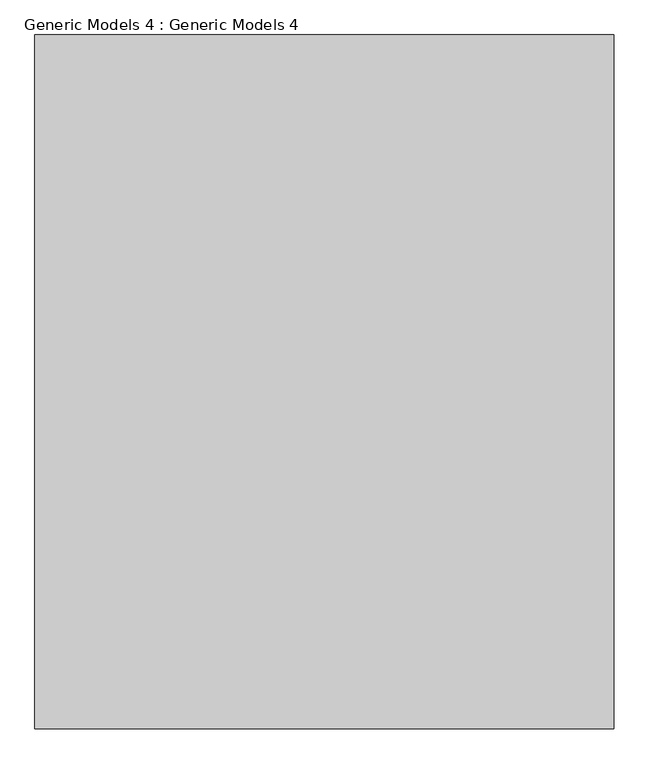
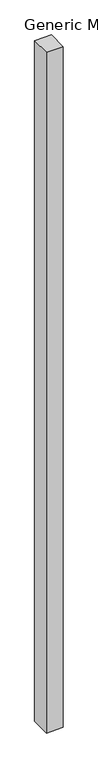
"""IFC4 building model written with IfcOpenShell, lengths in millimetres: proxy geometry, Generic Models 4 : Generic Models 4."""

from ifc_helpers import new_model, si_unit, frame, origin, place, context, project, spatial, polyline, outline, extrude, source, transform, mapped, element, save


def generic_models_4_generic_models_4_de7c2597(model_context):
    return source(origin(), model_context, "Body", "SweptSolid", [
        extrude(outline(polyline([(2801.4750471, -14078.0808221), (2801.4750471, -15453.557901), (1652.8739931, -15453.557901), (1652.8739931, -14078.0808221), (2801.4750471, -14078.0808221)])), frame((0.0, 0.0, 6522.896606), z_axis=(0.0, 0.0, 1.0), x_axis=(1.0, 0.0, 0.0)), (0.0, 0.0, 1.0), 48950.703394),
    ])


if __name__ == "__main__":
    model = new_model("IFC4")
    model_context = context("Model", 3, world=origin())
    ifc_project = project(units=[si_unit("LENGTHUNIT", "METRE", prefix="MILLI")], contexts=[model_context])
    site = spatial("IfcSite", under=ifc_project)
    building = spatial("IfcBuilding", under=site)
    placement = place(None, origin())
    generic_models_4_generic_models_4_shape = generic_models_4_generic_models_4_de7c2597(model_context)
    element("IfcBuildingElementProxy", 1, Name="Generic Models 4 : Generic Models 4", ObjectType="Generic Models 4 : Generic Models 4", at=placement, inside=building, context=model_context, shape_type="MappedRepresentation", body=[
        mapped(generic_models_4_generic_models_4_shape, transform((0.0, 0.0, 0.0), x_axis=(1.0, 0.0, 0.0), y_axis=(0.0, 1.0, 0.0), z_axis=(0.0, 0.0, 1.0))),
    ])
    save(model, "model.ifc")
